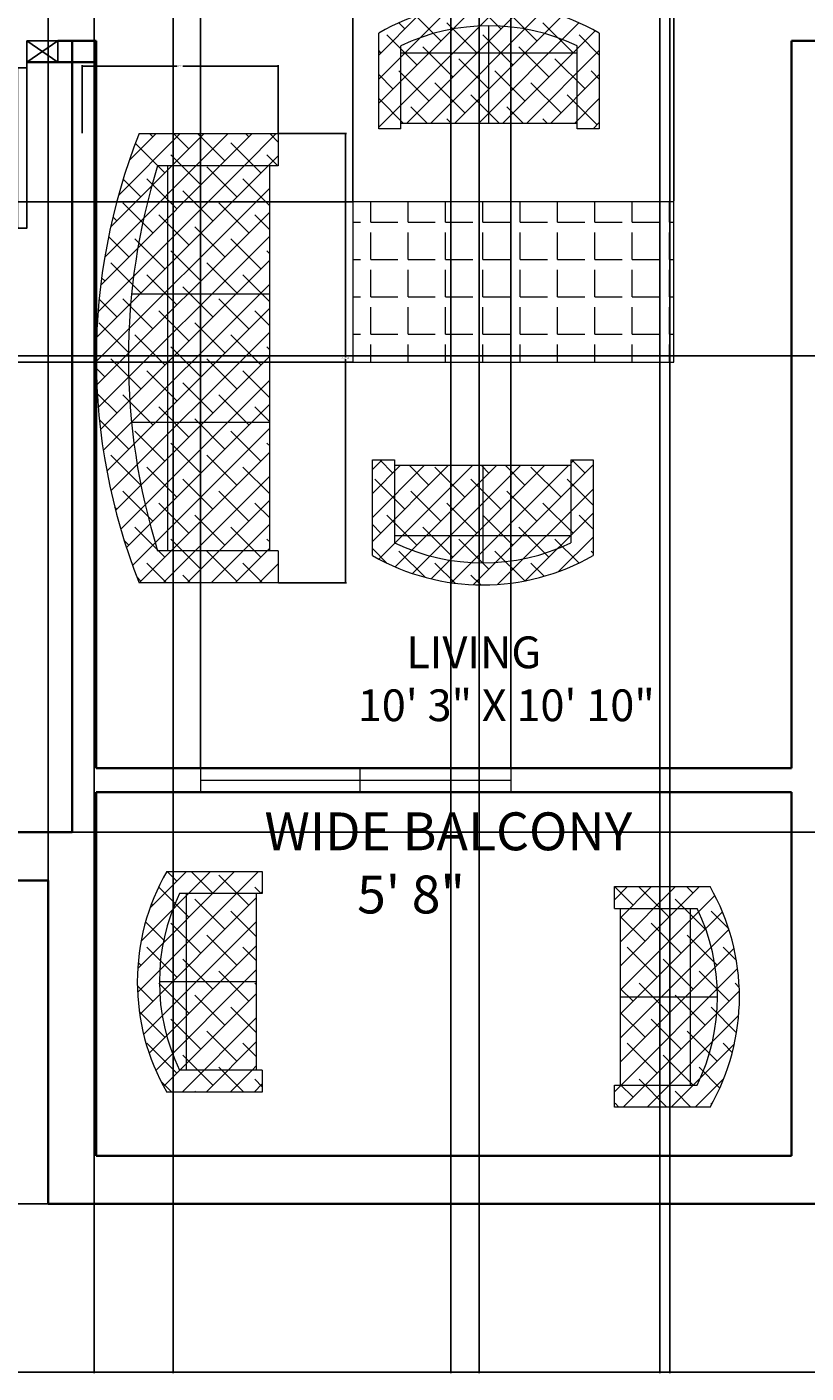
# Model space of a CAD drawing. Units: inches. Extents: x 2284228 to 3635239, y 3024422 to 8351872.
# Tile 2 of 7: x 3634888 to 3635034, y 8351218 to 8351470. Entities that reach past the tile are written whole.
import ezdxf

# ---------------------------------------------------------------- set-up
doc = ezdxf.new("R2010")
doc.units = ezdxf.units.IN
for name, color, linetype, lineweight in [('A-ANNO-DIMS', 2, 'Continuous', 18), ('A-AREA-IDEN', 7, 'Continuous', 18), ('A-DOOR', 4, 'Continuous', 25), ('A-FURN', 8, 'Continuous', 18), ('A-FURN-PATT', 9, 'Continuous', 13), ('A-GLAZ', 4, 'Continuous', 18), ('A-WALL', 7, 'Continuous', 35)]:
    doc.layers.add(name, color=color, linetype=linetype, lineweight=lineweight)
doc.styles.get("Standard").update_dxf_attribs({"font": 'arial.ttf'})
doc.dimstyles.get("Standard").update_dxf_attribs({"dimtxt": 0.18, "dimasz": 0.18, "dimexe": 0.18, "dimexo": 0.0625, "dimgap": 0.09, "dimtad": 0, "dimtih": 1, "dimtoh": 1, "dimdec": 4, "dimzin": 0, "dimdsep": 46, "dimtxsty": 'Standard', "dimcen": 0.09, "dimadec": 0, "dimazin": 0, "dimtfac": 1, "dimtdec": 4, "dimtofl": 0, "dimtmove": 0, "dimatfit": 3, "dimfxl": 1, "dimtolj": 1, "dimtzin": 0, "dimarcsym": 0})

# ---------------------------------------------------------------- blocks, each defined once
blk = doc.blocks.new('*U10')
for p, q in [((0, 0), (0, -5)), ((30, 0), (30, -5))]:
    blk.add_line(p, q)
blk.add_lwpolyline([(0, 0), (0, 30), (1.75, 30), (1.75, 0)], close=True)
blk.add_arc((0, 0), 30, 0, 90)
blk = doc.blocks.new('Sofa - Roundback 7 ft.')
for p, q in [((-12.00002, -32.4421), (-12.00003, -6.5971)), ((11.99997, -32.4421), (11.99998, -6.5971)), ((-36.000027, -34), (-36.000027, -11.4696)), ((35.99998, -34), (35.99998, -11.4696)), ((-35.999844, -13.3819), (35.9998, -13.3819)), ((-36.000027, -32.4421), (35.99998, -32.4421))]:
    blk.add_line(p, q)
for points in [[(-36.000027, -34), (-42.000027, -34), (-42.000027, -8)], [(41.99998, -8), (41.99998, -34), (35.99998, -34)]]:
    blk.add_lwpolyline(points)
for centre, radius, start, end in [((0, -114.25), 114.25, 68.43141, 111.5686), ((-0.00001, -127.1968), 121.1968, 72.72033, 107.2797)]:
    blk.add_arc(centre, radius, start, end)
blk = doc.blocks.new('Sofa - Roundback Loveseat 5 ft.')
for p, q in [((0, -32.44198), (0, -5.99998)), ((-24, -33.99998), (-24, -11.46958)), ((-23.9998, -13.38178), (23.99986, -13.38178)), ((24.00004, -33.99998), (24.00004, -11.46958)), ((-24, -32.44198), (24.00004, -32.44198))]:
    blk.add_line(p, q)
for points in [[(-24, -33.99998), (-30, -33.99998), (-30, -7.99998)], [(30.00004, -7.99998), (30.00004, -33.99998), (24.00004, -33.99998)]]:
    blk.add_lwpolyline(points)
for centre, radius, start, end in [((0, -60.24998), 60.24998, 60.13715, 119.8628), ((0, -61.38438), 55.38444, 64.32083, 115.6792)]:
    blk.add_arc(centre, radius, start, end)
blk = doc.blocks.new('*D36')
at = {"layer": 'A-ANNO-DIMS', "color": 0, "lineweight": -2, "transparency": 16777216}
for p, q in [((3634934.81, 8351450.22), (3634947.53, 8351450.22)), ((3634947.35, 8351450.04), (3634947.35, 8351408.4)), ((3634947.35, 8351366.4), (3634947.35, 8351408.03)), ((3634934.81, 8351366.22), (3634947.53, 8351366.22))]:
    blk.add_line(p, q, dxfattribs=at)
at = {"layer": 'A-ANNO-DIMS', "color": 0, "transparency": 16777216}
for points in [[(3634947.32, 8351450.04), (3634947.38, 8351450.04), (3634947.35, 8351450.22)], [(3634947.32, 8351366.4), (3634947.38, 8351366.4), (3634947.35, 8351366.22)]]:
    blk.add_solid(points, dxfattribs=at)
at = {"layer": 'Defpoints', "color": 0, "transparency": 16777216}
for p in [(3634934.75, 8351450.22), (3634947.35, 8351450.22), (3634934.75, 8351366.22)]:
    blk.add_point(p, dxfattribs=at)
at = {"layer": 'A-ANNO-DIMS', "color": 0, "transparency": 16777216, "insert": (3634947.35, 8351408.22), "char_height": 0.18, "attachment_point": 5}
blk.add_mtext('\\A1;SOFA 84 TYP.', dxfattribs=at)
blk = doc.blocks.new('*D37')
at = {"layer": 'A-ANNO-DIMS', "color": 0, "lineweight": -2, "transparency": 16777216}
for p, q in [((3634898.09, 8351450.28), (3634898.09, 8351463)), ((3634898.27, 8351462.82), (3634915.89, 8351462.82)), ((3634934.57, 8351462.82), (3634916.95, 8351462.82)), ((3634934.75, 8351450.28), (3634934.75, 8351463))]:
    blk.add_line(p, q, dxfattribs=at)
at = {"layer": 'A-ANNO-DIMS', "color": 0, "transparency": 16777216}
for points in [[(3634898.27, 8351462.85), (3634898.27, 8351462.79), (3634898.09, 8351462.82)], [(3634934.57, 8351462.85), (3634934.57, 8351462.79), (3634934.75, 8351462.82)]]:
    blk.add_solid(points, dxfattribs=at)
at = {"layer": 'Defpoints', "color": 0, "transparency": 16777216}
for p in [(3634898.09, 8351462.82), (3634898.09, 8351450.22), (3634934.75, 8351450.22)]:
    blk.add_point(p, dxfattribs=at)
at = {"layer": 'A-ANNO-DIMS', "color": 0, "transparency": 16777216, "insert": (3634916.42, 8351462.82), "char_height": 0.18, "attachment_point": 5}
blk.add_mtext('\\A1;37 TYP.', dxfattribs=at)
blk = doc.blocks.new('*D40')
at = {"layer": 'A-ANNO-DIMS', "color": 0, "lineweight": -2, "transparency": 16777216}
for p, q in [((3634700.92, 8351463.5), (3634700.92, 8351218.43)), ((3635206.75, 8351310.5), (3635206.75, 8351218.43)), ((3634701.1, 8351218.61), (3634953.44, 8351218.61)), ((3635206.57, 8351218.61), (3634954.23, 8351218.61))]:
    blk.add_line(p, q, dxfattribs=at)
at = {"layer": 'A-ANNO-DIMS', "color": 0, "transparency": 16777216}
for points in [[(3634701.1, 8351218.64), (3634701.1, 8351218.58), (3634700.92, 8351218.61)], [(3635206.57, 8351218.64), (3635206.57, 8351218.58), (3635206.75, 8351218.61)]]:
    blk.add_solid(points, dxfattribs=at)
at = {"layer": 'Defpoints', "color": 0, "transparency": 16777216}
for p in [(3634700.92, 8351463.56), (3635206.75, 8351310.56), (3635206.75, 8351218.61)]:
    blk.add_point(p, dxfattribs=at)
at = {"layer": 'A-ANNO-DIMS', "color": 0, "transparency": 16777216, "insert": (3634953.83, 8351218.61), "char_height": 0.18, "attachment_point": 5}
blk.add_mtext('\\A1;505.8', dxfattribs=at)
blk = doc.blocks.new('*D48')
at = {"layer": 'A-ANNO-DIMS', "color": 0, "lineweight": -2, "transparency": 16777216}
for p, q in [((3634891.69, 8351310.56), (3634669.29, 8351310.56)), ((3634669.47, 8351310.38), (3634669.47, 8351280.49)), ((3634669.47, 8351250.24), (3634669.47, 8351280.13)), ((3634891.69, 8351250.06), (3634669.29, 8351250.06))]:
    blk.add_line(p, q, dxfattribs=at)
at = {"layer": 'A-ANNO-DIMS', "color": 0, "transparency": 16777216}
for points in [[(3634669.44, 8351310.38), (3634669.5, 8351310.38), (3634669.47, 8351310.56)], [(3634669.44, 8351250.24), (3634669.5, 8351250.24), (3634669.47, 8351250.06)]]:
    blk.add_solid(points, dxfattribs=at)
at = {"layer": 'Defpoints', "color": 0, "transparency": 16777216}
for p in [(3634669.47, 8351310.56), (3634891.75, 8351310.56), (3634891.75, 8351250.06)]:
    blk.add_point(p, dxfattribs=at)
at = {"layer": 'A-ANNO-DIMS', "color": 0, "transparency": 16777216, "insert": (3634669.47, 8351280.31), "char_height": 0.18, "attachment_point": 5}
blk.add_mtext('\\A1;60.5', dxfattribs=at)
blk = doc.blocks.new('*D49')
at = {"layer": 'A-ANNO-DIMS', "color": 0, "lineweight": -2, "transparency": 16777216}
for p, q in [((3634891.75, 8351310.63), (3634891.75, 8351830.64)), ((3634891.93, 8351830.46), (3634965.47, 8351830.46)), ((3635039.57, 8351830.46), (3634966.03, 8351830.46)), ((3635039.75, 8351310.63), (3635039.75, 8351830.64))]:
    blk.add_line(p, q, dxfattribs=at)
at = {"layer": 'A-ANNO-DIMS', "color": 0, "transparency": 16777216}
for points in [[(3634891.93, 8351830.49), (3634891.93, 8351830.43), (3634891.75, 8351830.46)], [(3635039.57, 8351830.49), (3635039.57, 8351830.43), (3635039.75, 8351830.46)]]:
    blk.add_solid(points, dxfattribs=at)
at = {"layer": 'Defpoints', "color": 0, "transparency": 16777216}
for p in [(3635039.75, 8351830.46), (3634891.75, 8351310.56), (3635039.75, 8351310.56)]:
    blk.add_point(p, dxfattribs=at)
at = {"layer": 'A-ANNO-DIMS', "color": 0, "transparency": 16777216, "insert": (3634965.75, 8351830.46), "char_height": 0.18, "attachment_point": 5}
blk.add_mtext('\\A1;148', dxfattribs=at)
blk = doc.blocks.new('*D54')
at = {"layer": 'A-ANNO-DIMS', "color": 0, "lineweight": -2, "transparency": 16777216}
for p, q in [((3635006.17, 8351652.5), (3635006.17, 8351218.43)), ((3635036.17, 8351652.5), (3635036.17, 8351218.43)), ((3635006.35, 8351218.61), (3635020.95, 8351218.61)), ((3635035.99, 8351218.61), (3635021.38, 8351218.61))]:
    blk.add_line(p, q, dxfattribs=at)
at = {"layer": 'A-ANNO-DIMS', "color": 0, "transparency": 16777216}
for points in [[(3635006.35, 8351218.64), (3635006.35, 8351218.58), (3635006.17, 8351218.61)], [(3635035.99, 8351218.64), (3635035.99, 8351218.58), (3635036.17, 8351218.61)]]:
    blk.add_solid(points, dxfattribs=at)
at = {"layer": 'Defpoints', "color": 0, "transparency": 16777216}
for p in [(3635006.17, 8351652.56), (3635036.17, 8351652.56), (3635036.17, 8351218.61)]:
    blk.add_point(p, dxfattribs=at)
at = {"layer": 'A-ANNO-DIMS', "color": 0, "transparency": 16777216, "insert": (3635021.17, 8351218.61), "char_height": 0.18, "attachment_point": 5}
blk.add_mtext('\\A1;30', dxfattribs=at)
blk = doc.blocks.new('*D60')
at = {"layer": 'A-ANNO-DIMS', "color": 0, "lineweight": -2, "transparency": 16777216}
for p, q in [((3635099.17, 8351408.67), (3634669.29, 8351408.67)), ((3634669.47, 8351408.49), (3634669.47, 8351364.3)), ((3634669.47, 8351319.74), (3634669.47, 8351363.93)), ((3635099.17, 8351319.56), (3634669.29, 8351319.56))]:
    blk.add_line(p, q, dxfattribs=at)
at = {"layer": 'A-ANNO-DIMS', "color": 0, "transparency": 16777216}
for points in [[(3634669.44, 8351408.49), (3634669.5, 8351408.49), (3634669.47, 8351408.67)], [(3634669.44, 8351319.74), (3634669.5, 8351319.74), (3634669.47, 8351319.56)]]:
    blk.add_solid(points, dxfattribs=at)
at = {"layer": 'Defpoints', "color": 0, "transparency": 16777216}
for p in [(3635099.24, 8351408.67), (3634669.47, 8351319.56), (3635099.24, 8351319.56)]:
    blk.add_point(p, dxfattribs=at)
at = {"layer": 'A-ANNO-DIMS', "color": 0, "transparency": 16777216, "insert": (3634669.47, 8351364.12), "char_height": 0.18, "attachment_point": 5}
blk.add_mtext('\\A1;89.1', dxfattribs=at)
blk = doc.blocks.new('*D65')
at = {"layer": 'A-ANNO-DIMS', "color": 0, "lineweight": -2, "transparency": 16777216}
for p, q in [((3634900.35, 8351540.39), (3634900.35, 8351218.43)), ((3634972.35, 8351540.39), (3634972.35, 8351218.43)), ((3634900.53, 8351218.61), (3634936.13, 8351218.61)), ((3634972.17, 8351218.61), (3634936.57, 8351218.61))]:
    blk.add_line(p, q, dxfattribs=at)
at = {"layer": 'A-ANNO-DIMS', "color": 0, "transparency": 16777216}
for points in [[(3634900.53, 8351218.64), (3634900.53, 8351218.58), (3634900.35, 8351218.61)], [(3634972.17, 8351218.64), (3634972.17, 8351218.58), (3634972.35, 8351218.61)]]:
    blk.add_solid(points, dxfattribs=at)
at = {"layer": 'Defpoints', "color": 0, "transparency": 16777216}
for p in [(3634900.35, 8351540.45), (3634972.35, 8351540.45), (3634972.35, 8351218.61)]:
    blk.add_point(p, dxfattribs=at)
at = {"layer": 'A-ANNO-DIMS', "color": 0, "transparency": 16777216, "insert": (3634936.35, 8351218.61), "char_height": 0.18, "attachment_point": 5}
blk.add_mtext('\\A1;72', dxfattribs=at)
blk = doc.blocks.new('*D74')
at = {"layer": 'A-ANNO-DIMS', "color": 0, "lineweight": -2, "transparency": 16777216}
for p, q in [((3634920.21, 8351331.63), (3634920.21, 8351830.64)), ((3634920.39, 8351830.46), (3634948.84, 8351830.46)), ((3634978.09, 8351830.46), (3634949.63, 8351830.46)), ((3634978.27, 8351331.63), (3634978.27, 8351830.64))]:
    blk.add_line(p, q, dxfattribs=at)
at = {"layer": 'A-ANNO-DIMS', "color": 0, "transparency": 16777216}
for points in [[(3634920.39, 8351830.49), (3634920.39, 8351830.43), (3634920.21, 8351830.46)], [(3634978.09, 8351830.49), (3634978.09, 8351830.43), (3634978.27, 8351830.46)]]:
    blk.add_solid(points, dxfattribs=at)
at = {"layer": 'Defpoints', "color": 0, "transparency": 16777216}
for p in [(3634978.27, 8351830.46), (3634920.21, 8351331.56), (3634978.27, 8351331.56)]:
    blk.add_point(p, dxfattribs=at)
at = {"layer": 'A-ANNO-DIMS', "color": 0, "transparency": 16777216, "insert": (3634949.24, 8351830.46), "char_height": 0.18, "attachment_point": 5}
blk.add_mtext('\\A1;58.06', dxfattribs=at)
blk = doc.blocks.new('*D80')
at = {"layer": 'A-ANNO-DIMS', "color": 0, "lineweight": -2, "transparency": 16777216}
for p, q in [((3634948.75, 8351437.56), (3634948.75, 8351830.64)), ((3634948.93, 8351830.46), (3634978.53, 8351830.46)), ((3635008.57, 8351830.46), (3634978.97, 8351830.46)), ((3635008.75, 8351437.56), (3635008.75, 8351830.64))]:
    blk.add_line(p, q, dxfattribs=at)
at = {"layer": 'A-ANNO-DIMS', "color": 0, "transparency": 16777216}
for points in [[(3634948.93, 8351830.49), (3634948.93, 8351830.43), (3634948.75, 8351830.46)], [(3635008.57, 8351830.49), (3635008.57, 8351830.43), (3635008.75, 8351830.46)]]:
    blk.add_solid(points, dxfattribs=at)
at = {"layer": 'Defpoints', "color": 0, "transparency": 16777216}
for p in [(3635008.75, 8351830.46), (3634948.75, 8351437.49), (3635008.75, 8351437.49)]:
    blk.add_point(p, dxfattribs=at)
at = {"layer": 'A-ANNO-DIMS', "color": 0, "transparency": 16777216, "insert": (3634978.75, 8351830.46), "char_height": 0.18, "attachment_point": 5}
blk.add_mtext('\\A1;60', dxfattribs=at)
blk = doc.blocks.new('*D81')
at = {"layer": 'A-ANNO-DIMS', "color": 0, "lineweight": -2, "transparency": 16777216}
for p, q in [((3634948.68, 8351437.49), (3634669.29, 8351437.49)), ((3634669.47, 8351437.31), (3634669.47, 8351422.68)), ((3634669.47, 8351407.67), (3634669.47, 8351422.31)), ((3634948.68, 8351407.49), (3634669.29, 8351407.49))]:
    blk.add_line(p, q, dxfattribs=at)
at = {"layer": 'A-ANNO-DIMS', "color": 0, "transparency": 16777216}
for points in [[(3634669.44, 8351437.31), (3634669.5, 8351437.31), (3634669.47, 8351437.49)], [(3634669.44, 8351407.67), (3634669.5, 8351407.67), (3634669.47, 8351407.49)]]:
    blk.add_solid(points, dxfattribs=at)
at = {"layer": 'Defpoints', "color": 0, "transparency": 16777216}
for p in [(3634669.47, 8351437.49), (3634948.75, 8351437.49), (3634948.75, 8351407.49)]:
    blk.add_point(p, dxfattribs=at)
at = {"layer": 'A-ANNO-DIMS', "color": 0, "transparency": 16777216, "insert": (3634669.47, 8351422.49), "char_height": 0.18, "attachment_point": 5}
blk.add_mtext('\\A1;30', dxfattribs=at)
blk = doc.blocks.new('*D82')
at = {"layer": 'A-ANNO-DIMS', "color": 0, "lineweight": -2, "transparency": 16777216}
for p, q in [((3634915.11, 8351783.43), (3634915.11, 8351218.43)), ((3634967.04, 8351783.43), (3634967.04, 8351218.43)), ((3634915.29, 8351218.61), (3634940.68, 8351218.61)), ((3634966.86, 8351218.61), (3634941.47, 8351218.61))]:
    blk.add_line(p, q, dxfattribs=at)
at = {"layer": 'A-ANNO-DIMS', "color": 0, "transparency": 16777216}
for points in [[(3634915.29, 8351218.64), (3634915.29, 8351218.58), (3634915.11, 8351218.61)], [(3634966.86, 8351218.64), (3634966.86, 8351218.58), (3634967.04, 8351218.61)]]:
    blk.add_solid(points, dxfattribs=at)
at = {"layer": 'Defpoints', "color": 0, "transparency": 16777216}
for p in [(3634915.11, 8351783.5), (3634967.04, 8351783.5), (3634967.04, 8351218.61)]:
    blk.add_point(p, dxfattribs=at)
at = {"layer": 'A-ANNO-DIMS', "color": 0, "transparency": 16777216, "insert": (3634941.08, 8351218.61), "char_height": 0.18, "attachment_point": 5}
blk.add_mtext('\\A1;51.94', dxfattribs=at)
blk = doc.blocks.new('*D83')
at = {"layer": 'A-ANNO-DIMS', "color": 0, "lineweight": -2, "transparency": 16777216}
for p, q in [((3634967.04, 8351783.43), (3634967.04, 8351218.43)), ((3635008.03, 8351783.43), (3635008.03, 8351218.43)), ((3634967.22, 8351218.61), (3634987.14, 8351218.61)), ((3635007.85, 8351218.61), (3634987.93, 8351218.61))]:
    blk.add_line(p, q, dxfattribs=at)
at = {"layer": 'A-ANNO-DIMS', "color": 0, "transparency": 16777216}
for points in [[(3634967.22, 8351218.64), (3634967.22, 8351218.58), (3634967.04, 8351218.61)], [(3635007.85, 8351218.64), (3635007.85, 8351218.58), (3635008.03, 8351218.61)]]:
    blk.add_solid(points, dxfattribs=at)
at = {"layer": 'Defpoints', "color": 0, "transparency": 16777216}
for p in [(3634967.04, 8351783.5), (3635008.03, 8351783.5), (3635008.03, 8351218.61)]:
    blk.add_point(p, dxfattribs=at)
at = {"layer": 'A-ANNO-DIMS', "color": 0, "transparency": 16777216, "insert": (3634987.54, 8351218.61), "char_height": 0.18, "attachment_point": 5}
blk.add_mtext('\\A1;40.98', dxfattribs=at)

msp = doc.modelspace()

# ---------------------------------------------------------------- hatches: boundary and pattern name
at = {"layer": 'A-FURN-PATT'}
h = msp.add_hatch(dxfattribs=at)
h.set_pattern_fill('ANSI38', color=256)
h.paths.add_polyline_path([(3634930.7271, 8351308.1081), (3634917.6211, 8351308.1081), (3634917.6211, 8351291.6054), (3634930.7271, 8351291.6054)], flags=17)
h.paths.add_polyline_path([(3634917.6211, 8351308.1081), (3634916.3066, 8351308.1081, 0.11251889), (3634912.5453, 8351291.6054), (3634917.6211, 8351291.6054)], flags=17)
h.paths.add_polyline_path([(3634930.7271, 8351291.6054), (3634917.6211, 8351291.6054), (3634917.6211, 8351275.1027), (3634930.7271, 8351275.1027)], flags=17)
h.paths.add_polyline_path([(3634917.6211, 8351291.6054), (3634912.5453, 8351291.6054, 0.11251869), (3634916.3066, 8351275.1027), (3634917.6211, 8351275.1027)], flags=17)
h.paths.add_polyline_path([(3634931.7984, 8351312.2337), (3634913.9206, 8351312.2337, 0.26666697), (3634913.9206, 8351270.977), (3634931.7984, 8351270.977), (3634931.7984, 8351275.1027), (3634916.3066, 8351275.1027, -0.11251869), (3634912.5453, 8351291.6054, -0.11251889), (3634916.3066, 8351308.1081), (3634931.7984, 8351308.1081)])
h.paths.add_polyline_path([(3635011.8389, 8351305.2814), (3634998.7329, 8351305.2814), (3634998.7329, 8351288.7787), (3635011.8389, 8351288.7787)], flags=17)
h.paths.add_polyline_path([(3635011.8389, 8351288.7787), (3634998.7329, 8351288.7787), (3634998.7329, 8351272.276), (3635011.8389, 8351272.276)], flags=17)
h.paths.add_polyline_path([(3635016.9148, 8351288.7787), (3635011.8389, 8351288.7787), (3635011.8389, 8351272.276), (3635013.1534, 8351272.276, 0.11251889)], flags=17)
h.paths.add_polyline_path([(3635013.1534, 8351305.2814), (3635011.8389, 8351305.2814), (3635011.8389, 8351288.7787), (3635016.9148, 8351288.7787, 0.11251869)], flags=17)
h.paths.add_polyline_path([(3635015.5395, 8351309.407), (3634997.6616, 8351309.407), (3634997.6616, 8351305.2814), (3635013.1534, 8351305.2814, -0.11251869), (3635016.9148, 8351288.7787, -0.11251889), (3635013.1534, 8351272.276), (3634997.6616, 8351272.276), (3634997.6616, 8351268.1503), (3635015.5395, 8351268.1503, 0.26666697)])
h.paths.add_polyline_path([(3635065.1595, 8351552.9755), (3635052.0535, 8351552.9755), (3635052.0535, 8351536.4728), (3635065.1595, 8351536.4728)], flags=17)
h.paths.add_polyline_path([(3635065.1595, 8351536.4728), (3635052.0535, 8351536.4728), (3635052.0535, 8351519.9701), (3635065.1595, 8351519.9701)], flags=17)
h.paths.add_polyline_path([(3635052.0535, 8351536.4728), (3635046.9776, 8351536.4728, 0.11251869), (3635050.739, 8351519.9701), (3635052.0535, 8351519.9701)], flags=17)
h.paths.add_polyline_path([(3635052.0535, 8351552.9755), (3635050.739, 8351552.9755, 0.11251889), (3635046.9776, 8351536.4728), (3635052.0535, 8351536.4728)], flags=17)
h.paths.add_polyline_path([(3635066.2308, 8351519.9701), (3635050.739, 8351519.9701, -0.11251869), (3635046.9776, 8351536.4728, -0.11251889), (3635050.739, 8351552.9755), (3635066.2308, 8351552.9755), (3635066.2308, 8351557.1011), (3635048.3529, 8351557.1011, 0.26666697), (3635048.3529, 8351515.8444), (3635066.2308, 8351515.8444)])
h.paths.add_polyline_path([(3635177.7039, 8351552.9754), (3635164.5979, 8351552.9754), (3635164.5979, 8351536.4728), (3635177.7039, 8351536.4728)], flags=17)
h.paths.add_polyline_path([(3635179.0184, 8351552.9754), (3635177.7039, 8351552.9754), (3635177.7039, 8351536.4728), (3635182.7797, 8351536.4728, 0.11251869)], flags=17)
h.paths.add_polyline_path([(3635177.7039, 8351536.4728), (3635164.5979, 8351536.4728), (3635164.5979, 8351519.9701), (3635177.7039, 8351519.9701)], flags=17)
h.paths.add_polyline_path([(3635182.7797, 8351536.4728), (3635177.7039, 8351536.4728), (3635177.7039, 8351519.9701), (3635179.0184, 8351519.9701, 0.11251889)], flags=17)
h.paths.add_polyline_path([(3635181.4045, 8351557.1011), (3635163.5266, 8351557.1011), (3635163.5266, 8351552.9754), (3635179.0184, 8351552.9754, -0.11251869), (3635182.7797, 8351536.4728, -0.11251889), (3635179.0184, 8351519.9701), (3635163.5266, 8351519.9701), (3635163.5266, 8351515.8444), (3635181.4045, 8351515.8444, 0.26666697)])
h.paths.add_polyline_path([(3635154.1523, 8351500.1911), (3635130.1523, 8351500.1911), (3635130.1523, 8351481.1309), (3635154.1523, 8351481.1309)], flags=17)
h.paths.add_polyline_path([(3635130.1523, 8351500.1911), (3635106.1523, 8351500.1911), (3635106.1523, 8351481.1309), (3635130.1523, 8351481.1309)], flags=17)
h.paths.add_polyline_path([(3635106.1523, 8351500.1911), (3635082.1523, 8351500.1911), (3635082.1523, 8351481.1309), (3635106.1523, 8351481.1309)], flags=17)
h.paths.add_polyline_path([(3635106.1523, 8351481.1309), (3635082.1523, 8351481.1309), (3635082.1523, 8351479.2191, 0.05064665), (3635106.1523, 8351474.3445)], flags=17)
h.paths.add_polyline_path([(3635130.1523, 8351481.1309), (3635106.1523, 8351481.1309), (3635106.1523, 8351474.3461), (3635106.1523, 8351474.3445, 0.04962821), (3635130.1523, 8351474.3445)], flags=17)
h.paths.add_polyline_path([(3635154.1523, 8351479.2191), (3635154.1523, 8351481.1309), (3635130.1523, 8351481.1309), (3635130.1523, 8351474.3445, 0.05064665)], flags=17)
h.paths.add_polyline_path([(3635160.1523, 8351475.749), (3635160.1523, 8351501.749), (3635154.1523, 8351501.749), (3635154.1523, 8351479.2191, -0.15194781), (3635082.1523, 8351479.2191), (3635082.1523, 8351501.749), (3635076.1523, 8351501.749), (3635076.1523, 8351475.749, 0.19047621)])
h = msp.add_hatch(dxfattribs=at)
h.set_pattern_fill('ANSI38', color=256)
h.paths.add_polyline_path([(3634933.1946, 8351444.2171), (3634914.1344, 8351444.2171), (3634914.1344, 8351420.2171), (3634933.1946, 8351420.2171)], flags=17)
h.paths.add_polyline_path([(3634933.1946, 8351420.2171), (3634914.1344, 8351420.2171), (3634914.1344, 8351396.2171), (3634933.1946, 8351396.2171)], flags=17)
h.paths.add_polyline_path([(3634933.1946, 8351396.2171), (3634914.1344, 8351396.2171), (3634914.1344, 8351372.2171), (3634933.1946, 8351372.2171)], flags=17)
h.paths.add_polyline_path([(3634914.1344, 8351396.2171), (3634907.348, 8351396.2171, 0.05064665), (3634912.2226, 8351372.2171), (3634914.1344, 8351372.2171)], flags=17)
h.paths.add_polyline_path([(3634914.1344, 8351420.2171), (3634907.348, 8351420.2171, 0.04962821), (3634907.348, 8351396.2171), (3634914.1344, 8351396.2171)], flags=17)
h.paths.add_polyline_path([(3634914.1344, 8351444.2171), (3634912.2226, 8351444.2171, 0.05064665), (3634907.348, 8351420.2171), (3634914.1344, 8351420.2171)], flags=17)
h.paths.add_polyline_path([(3634934.7525, 8351450.2171), (3634908.7525, 8351450.2171, 0.19047621), (3634908.7525, 8351366.2171), (3634934.7525, 8351366.2171), (3634934.7525, 8351372.2171), (3634912.2226, 8351372.2171, -0.05064665), (3634907.348, 8351396.2171, -0.10052754), (3634912.2226, 8351444.2171), (3634934.7525, 8351444.2171)])
h.paths.add_polyline_path([(3634993.654, 8351371.3187), (3634993.654, 8351389.1966), (3634989.5284, 8351389.1966), (3634989.5284, 8351373.7048, -0.22792319), (3634956.523, 8351373.7048), (3634956.523, 8351389.1966), (3634952.3973, 8351389.1966), (3634952.3973, 8351371.3187, 0.26666697)])
h.paths.add_polyline_path([(3634989.5284, 8351373.7048), (3634989.5284, 8351375.0193), (3634973.0257, 8351375.0193), (3634973.0257, 8351369.9434, 0.11251869)], flags=17)
h.paths.add_polyline_path([(3634973.0257, 8351375.0193), (3634956.523, 8351375.0193), (3634956.523, 8351373.7048, 0.11251889), (3634973.0257, 8351369.9434)], flags=17)
h.paths.add_polyline_path([(3634973.0257, 8351388.1253), (3634956.523, 8351388.1253), (3634956.523, 8351375.0193), (3634973.0257, 8351375.0193)], flags=17)
h.paths.add_polyline_path([(3634989.5284, 8351388.1253), (3634973.0257, 8351388.1253), (3634973.0257, 8351375.0193), (3634989.5284, 8351375.0193)], flags=17)
h.paths.add_polyline_path([(3634990.6934, 8351465.3078), (3634974.1907, 8351465.3078), (3634974.1907, 8351452.2018), (3634990.6934, 8351452.2018)], flags=17)
h.paths.add_polyline_path([(3634974.1907, 8351465.3078), (3634957.688, 8351465.3078), (3634957.688, 8351452.2018), (3634974.1907, 8351452.2018)], flags=17)
h.paths.add_polyline_path([(3634974.1907, 8351470.3836, 0.11251869), (3634957.688, 8351466.6223), (3634957.688, 8351465.3078), (3634974.1907, 8351465.3078)], flags=17)
h.paths.add_polyline_path([(3634974.1907, 8351470.3836), (3634974.1907, 8351465.3078), (3634990.6934, 8351465.3078), (3634990.6934, 8351466.6222, 0.11251889)], flags=17)
h.paths.add_polyline_path([(3634953.5624, 8351469.0083), (3634953.5624, 8351451.1305), (3634957.688, 8351451.1305), (3634957.688, 8351466.6223, -0.11251869), (3634974.1907, 8351470.3836, -0.11251889), (3634990.6934, 8351466.6222), (3634990.6934, 8351451.1305), (3634994.819, 8351451.1305), (3634994.819, 8351469.0083, 0.26666697)])
h = msp.add_hatch(dxfattribs=at)
h.set_pattern_fill('ANGLE', color=256)
h.set_pattern_definition([(0, (0, 0), (0, 6.985), [5.08, -1.905]), (90, (0, 0), (-6.985, 4e-16), [5.08, -1.905])])
h.paths.add_polyline_path([(3635008.7462, 8351437.4931), (3634948.7462, 8351437.4931), (3634948.7462, 8351407.4931), (3635008.7462, 8351407.4931)])

# ---------------------------------------------------------------- linework, layer by layer
at = {"layer": 'A-DOOR'}
for p, q in [((3634887.7742, 8351463.5627), (3634893.585, 8351467.5627)), ((3634887.7742, 8351467.5472), (3634893.585, 8351467.5627)), ((3634887.7742, 8351467.5472), (3634893.585, 8351463.5627)), ((3634893.585, 8351467.5627), (3634893.585, 8351463.5627))]:
    msp.add_line(p, q, dxfattribs=at)
at = {"layer": 'A-FURN'}
for p, q in [((3634948.7462, 8351437.4931), (3634948.7462, 8351407.4931)), ((3635008.7462, 8351437.4931), (3634948.7462, 8351437.4931)), ((3635008.7462, 8351407.4931), (3635008.7462, 8351437.4931)), ((3634948.7462, 8351407.4931), (3635008.7462, 8351407.4931))]:
    msp.add_line(p, q, dxfattribs=at)
at = {"layer": 'A-GLAZ'}
for p, q in [((3634920.2105, 8351331.5627), (3634920.2105, 8351327.0627)), ((3634950.0122, 8351331.5627), (3634950.0122, 8351327.0627)), ((3634978.266, 8351331.5627), (3634978.266, 8351327.0627)), ((3634920.2105, 8351329.3127), (3634978.266, 8351329.3127))]:
    msp.add_line(p, q, dxfattribs=at)
at = {"layer": 'A-WALL'}
for p, q in [((3634893.585, 8351467.5627), (3634900.7525, 8351467.5627)), ((3634896.2525, 8351319.5627), (3634896.2525, 8351467.5627)), ((3634900.7525, 8351331.5627), (3634900.7525, 8351467.5627)), ((3635030.7525, 8351467.5627), (3635031.7525, 8351467.5627)), ((3635030.7525, 8351331.5627), (3635030.7525, 8351467.5627)), ((3635031.7525, 8351467.5627), (3635197.7525, 8351467.5627)), ((3634887.7742, 8351463.5627), (3634900.7525, 8351463.5627)), ((3634900.7525, 8351331.5627), (3635030.7525, 8351331.5627)), ((3634900.7525, 8351259.0627), (3634900.7525, 8351327.0627)), ((3634900.7525, 8351327.0627), (3635030.7525, 8351327.0627)), ((3635030.7525, 8351259.0627), (3635030.7525, 8351327.0627)), ((3634752.2525, 8351319.5627), (3634896.2525, 8351319.5627)), ((3634752.2525, 8351319.5627), (3634896.2525, 8351319.5627)), ((3634743.2525, 8351310.5627), (3634891.7525, 8351310.5627)), ((3634891.7525, 8351250.0627), (3634891.7525, 8351310.5627)), ((3634900.7525, 8351259.0627), (3635030.7525, 8351259.0627)), ((3634891.7525, 8351250.0627), (3635039.7525, 8351250.0627))]:
    msp.add_line(p, q, dxfattribs=at)

# ---------------------------------------------------------------- block references
at = {"layer": 'A-DOOR', "rotation": 180}
msp.add_blockref('*U10', (3634887.7742, 8351462.5472), dxfattribs=at)
at = {"layer": 'A-FURN', "xscale": 0.6876111649018397, "yscale": 0.6876111649018397, "zscale": 0.6876111649018397}
msp.add_blockref('Sofa - Roundback Loveseat 5 ft.', (3634974.1907, 8351474.5092), dxfattribs=at)
at = {"layer": 'A-FURN', "rotation": 89.99999999999999}
msp.add_blockref('Sofa - Roundback 7 ft.', (3634900.7525, 8351408.2171), dxfattribs=at)
at = {"layer": 'A-FURN', "xscale": 0.6876111649018397, "yscale": 0.6876111649018397, "zscale": 0.6876111649018397}
for p, rotation in [((3634973.0257, 8351365.8178), 180), ((3634908.4197, 8351291.6054), 89.99999999999999), ((3635021.0404, 8351288.7787), 270)]:
    msp.add_blockref('Sofa - Roundback Loveseat 5 ft.', p, dxfattribs=dict(at, rotation=rotation))

# ---------------------------------------------------------------- texts
at = {"layer": 'A-AREA-IDEN', "attachment_point": 1}
for s, width, gutter_width, insert, char_height in [('        LIVING \\P   10\' 3" X 10\' 10"', 331.491197, 29.698, (3634944.1971, 8351356.1853), 5.939604), ('   WIDE BALCONY\\P           5\' 8"', 177.180538, 35.4278, (3634925.7108, 8351323.2833), 7.085555)]:
    msp.add_mtext_dynamic_manual_height_columns(s, width=width, gutter_width=gutter_width, heights=[0], dxfattribs=dict(at, insert=insert, char_height=char_height))

# ---------------------------------------------------------------- dimensions: what is measured, and where the dimension line sits
at = {"layer": 'A-ANNO-DIMS'}
for base, p1, p2, override, picture, middle in [((3635039.7525, 8351830.4618), (3634891.7525, 8351310.5627), (3635039.7525, 8351310.5627), {"dimdec": 0, "dimlfac": 1, "dimrnd": 0, "dimzin": 0, "dimdsep": 46, "dimlunit": 2}, '*D49', (3634965.7525, 8351830.4618)), ((3634978.266, 8351830.4618), (3634920.2105, 8351331.5627), (3634978.266, 8351331.5627), {"dimdec": 2, "dimlfac": 1, "dimrnd": 0, "dimzin": 0, "dimdsep": 46, "dimlunit": 2}, '*D74', (3634949.2383, 8351830.4618)), ((3635008.7462, 8351830.4618), (3634948.7462, 8351437.4931), (3635008.7462, 8351437.4931), {"dimdec": 0, "dimlfac": 1, "dimrnd": 0, "dimzin": 0, "dimdsep": 46, "dimlunit": 2}, '*D80', (3634978.7462, 8351830.4618)), ((3634967.0447, 8351218.6127), (3634915.1056, 8351783.4971), (3634967.0447, 8351783.4971), {"dimdec": 2, "dimlfac": 1, "dimrnd": 0, "dimzin": 0, "dimdsep": 46, "dimlunit": 2}, '*D82', (3634941.0752, 8351218.6127)), ((3635008.0257, 8351218.6127), (3634967.0447, 8351783.4971), (3635008.0257, 8351783.4971), {"dimdec": 2, "dimlfac": 1, "dimrnd": 0, "dimzin": 0, "dimdsep": 46, "dimlunit": 2}, '*D83', (3634987.5352, 8351218.6127)), ((3635036.1658, 8351218.6127), (3635006.1658, 8351652.5627), (3635036.1658, 8351652.5627), {"dimdec": 0, "dimlfac": 1, "dimrnd": 0, "dimzin": 0, "dimdsep": 46, "dimlunit": 2}, '*D54', (3635021.1658, 8351218.6127)), ((3634972.3485, 8351218.6127), (3634900.3485, 8351540.4517), (3634972.3485, 8351540.4517), {"dimdec": 0, "dimlfac": 1, "dimrnd": 0, "dimzin": 0, "dimdsep": 46, "dimlunit": 2}, '*D65', (3634936.3485, 8351218.6127)), ((3635206.7525, 8351218.6127), (3634700.915, 8351463.5627), (3635206.7525, 8351310.5627), {"dimdec": 1, "dimlfac": 1, "dimrnd": 0, "dimzin": 0, "dimdsep": 46, "dimlunit": 2}, '*D40', (3634953.8337, 8351218.6127))]:
    dim = msp.add_linear_dim(base=base, p1=p1, p2=p2, dimstyle='Standard', override=override, dxfattribs=at)
    dim.commit()
    dim.dimension.update_dxf_attribs({"geometry": picture, "text_midpoint": middle})
for base, p1, p2, angle, text, picture, middle in [((3634898.0858, 8351462.8171), (3634934.7525, 8351450.2171), (3634898.0858, 8351450.2171), 180, '<> TYP.', '*D37', (3634916.4191, 8351462.8171)), ((3634947.3525, 8351450.2171), (3634934.7525, 8351366.2171), (3634934.7525, 8351450.2171), 90, 'SOFA <> TYP.', '*D36', (3634947.3525, 8351408.2171))]:
    dim = msp.add_linear_dim(base=base, p1=p1, p2=p2, angle=angle, text=text, dimstyle='Standard', override={"dimdec": 0, "dimlfac": 1, "dimrnd": 0, "dimzin": 0, "dimdsep": 46, "dimlunit": 2}, dxfattribs=at)
    dim.commit()
    dim.dimension.update_dxf_attribs({"geometry": picture, "text_midpoint": middle})
for base, p1, p2, override, picture, middle in [((3634669.465, 8351437.4931), (3634948.7462, 8351407.4931), (3634948.7462, 8351437.4931), {"dimdec": 0, "dimlfac": 1, "dimrnd": 0, "dimzin": 0, "dimdsep": 46, "dimlunit": 2}, '*D81', (3634669.465, 8351422.4931)), ((3634669.465, 8351319.5627), (3635099.2364, 8351408.6677), (3635099.2364, 8351319.5627), {"dimdec": 1, "dimlfac": 1, "dimrnd": 0, "dimzin": 0, "dimdsep": 46, "dimlunit": 2}, '*D60', (3634669.465, 8351364.1152)), ((3634669.465, 8351310.5627), (3634891.7525, 8351250.0627), (3634891.7525, 8351310.5627), {"dimdec": 1, "dimlfac": 1, "dimrnd": 0, "dimzin": 0, "dimdsep": 46, "dimlunit": 2}, '*D48', (3634669.465, 8351280.3127))]:
    dim = msp.add_linear_dim(base=base, p1=p1, p2=p2, angle=90, dimstyle='Standard', override=override, dxfattribs=at)
    dim.commit()
    dim.dimension.update_dxf_attribs({"geometry": picture, "text_midpoint": middle})

doc.saveas('drawing.dxf')
